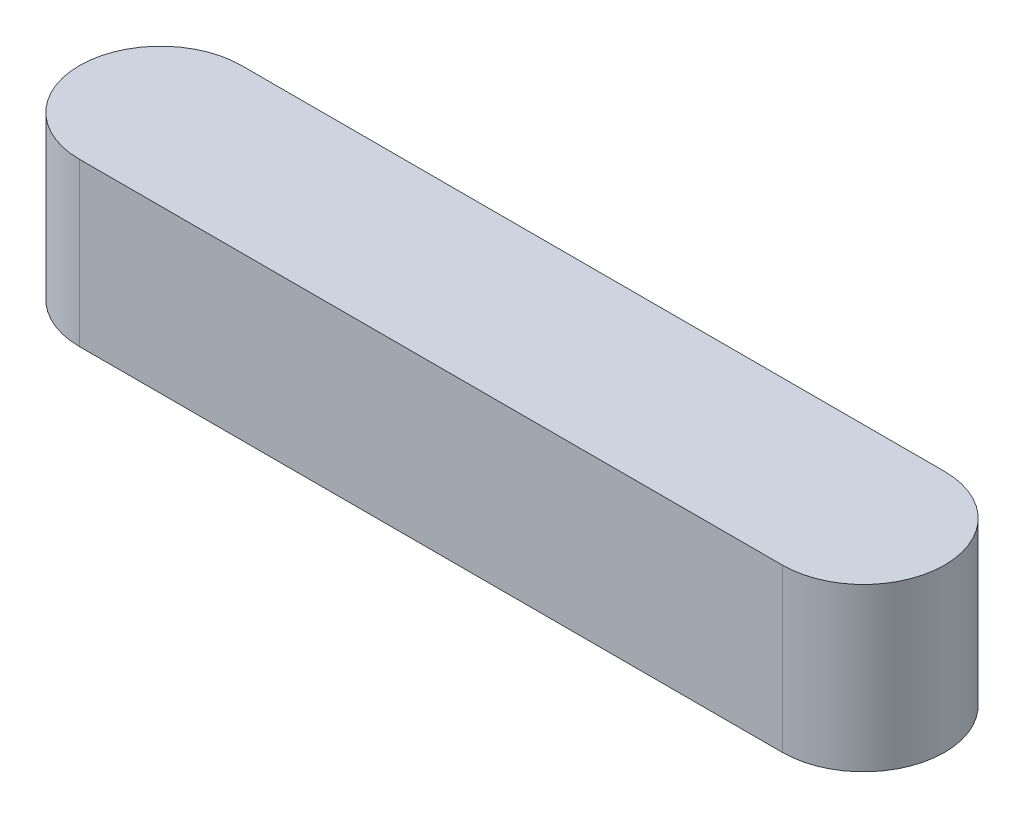
SolidWorks part; units mm, degrees
material "Plain Carbon Steel"
ref_plane "Front Plane" through (0, 0, 0) normal (0, 0, 1) x (1, 0, 0)
ref_plane "Top Plane" through (0, 0, 0) normal (0, 1, 0) x (1, 0, 0)
ref_plane "Right Plane" through (0, 0, 0) normal (1, 0, 0) x (0, 0, -1)
sketch "Key Profile Slot 6x32" plane through (0, 0, 0) normal (0, 1, 0) x (1, 0, 0)
  line L0 (-13, 0) -> (13, 0) construction
  line L1 (-13, 3) -> (13, 3)
  line L2 (-13, -3) -> (13, -3)
  arc A0 (-13, 3) -> (-13, -3) centre (-13, 0) ccw
  arc A1 (13, -3) -> (13, 3) centre (13, 0) ccw
  point P2 (0, 0)
  dimension "D2" = 3
  dimension "D1" = 26
extrude "Key Body 6x6x32" add sketch "Key Profile Slot 6x32" along normal blind 6
